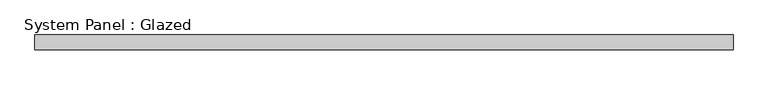
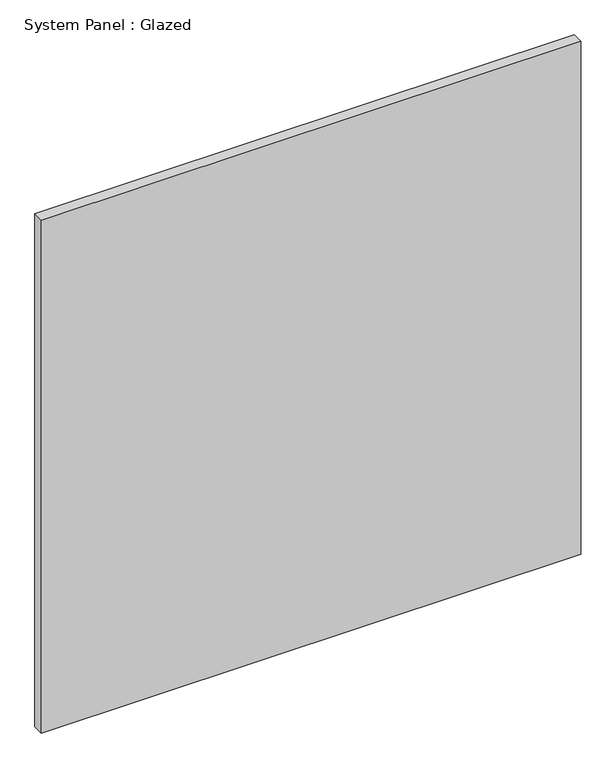
"""IFC4 building model written with IfcOpenShell, lengths in millimetres: plate geometry, System Panel : Glazed."""

from ifc_helpers import new_model, si_unit, origin, origin_with_axes, place, context, project, spatial, polyline, outline, extrude, source, transform, mapped, element, save


def system_panel_glazed_576ad081(model_context):
    return source(origin(), model_context, "Body", "SweptSolid", [
        extrude(outline(polyline([(596.6666667, -49.5), (-596.6666667, -49.5), (-596.6666667, -24.5), (596.6666667, -24.5), (596.6666667, -49.5)])), origin_with_axes(), (0.0, 0.0, 1.0), 1200.0),
    ])


if __name__ == "__main__":
    model = new_model("IFC4")
    model_context = context("Model", 3, world=origin())
    ifc_project = project(units=[si_unit("LENGTHUNIT", "METRE", prefix="MILLI")], contexts=[model_context])
    site = spatial("IfcSite", under=ifc_project)
    building = spatial("IfcBuilding", under=site)
    placement = place(None, origin())
    system_panel_glazed_shape = system_panel_glazed_576ad081(model_context)
    element("IfcPlate", 1, ObjectType="System Panel : Glazed", at=placement, inside=building, context=model_context, shape_type="MappedRepresentation", body=[
        mapped(system_panel_glazed_shape, transform((0.0, 0.0, 0.0), x_axis=(1.0, 0.0, 0.0), y_axis=(0.0, 1.0, 0.0), z_axis=(0.0, 0.0, 1.0))),
    ])
    save(model, "model.ifc")

# Revit data of these elements
# Type "System Panel : Glazed"
#   Keynote = "H11"
#   Construction Type Id = "GSP4R"
#   Analytic Construction = "1/8 in Pilkington single glazing"
#   Visual Light Transmittance = 0.9
#   Solar Heat Gain Coefficient = 0.86
#   Heat Transfer Coefficient (U) = 6.7069 W/(m²·K)
#   Define Thermal Properties by = 1
# Element 1 (IfcPlate, "System Panel : Glazed")
#   Materials on its faces: "Glass"
# Materials
#   "Glass": class "Glass", colour RGB 0 128 192, transparency 0.9, Description = "Soda Lime Glass", Cost = 0
